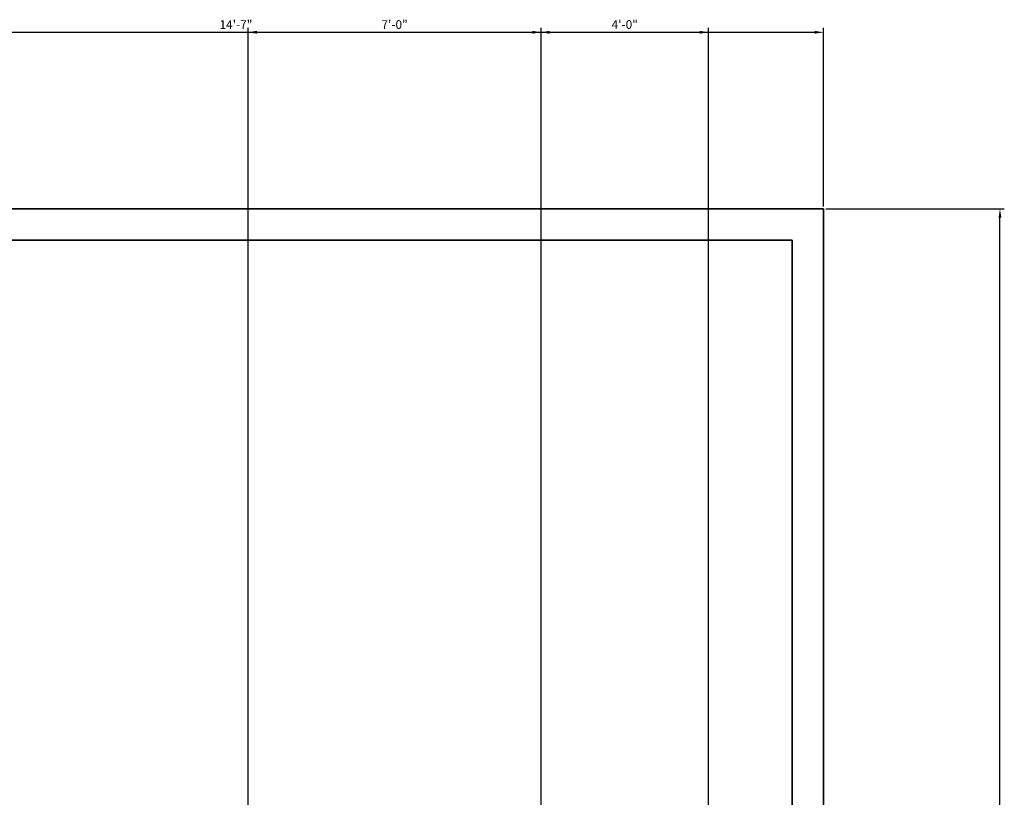
# Model space of a CAD drawing. Units: inches. Extents: x 3412 to 4225, y 13529 to 14581.
# Tile 7 of 7: x 3943 to 4225, y 14358 to 14581. Entities that reach past the tile are written whole.
import ezdxf

# ---------------------------------------------------------------- set-up
doc = ezdxf.new("R2010")
doc.units = ezdxf.units.IN
doc.layers.add('A-ANNO-DIMS', color=2, linetype='Continuous', lineweight=13)
doc.layers.add('C-SITE-WALL', color=7, linetype='Continuous', lineweight=35)
doc.styles.get("Standard").update_dxf_attribs({"font": 'arial.ttf'})
doc.dimstyles.new('ISO-25', dxfattribs={"dimtxt": 2.5, "dimasz": 2.5, "dimexe": 1.25, "dimexo": 0.625, "dimtad": 1, "dimdec": 0, "dimlunit": 3, "dimtxsty": 'Standard', "dimcen": 2.5, "dimadec": 0, "dimazin": 0, "dimtfac": 1, "dimtdec": 0, "dimtmove": 0, "dimatfit": 3, "dimfxl": 1, "dimarcsym": 0})

# ---------------------------------------------------------------- blocks, each defined once
blk = doc.blocks.new('*D56')
at = {"layer": 'A-ANNO-DIMS', "color": 0, "lineweight": -2, "transparency": 16777216}
for p, q in [((3468.36, 14527.06), (3468.36, 14578.28)), ((4173.36, 14527.06), (4173.36, 14578.28)), ((3470.86, 14577.03), (4170.86, 14577.03))]:
    blk.add_line(p, q, dxfattribs=at)
at = {"layer": 'A-ANNO-DIMS', "color": 0, "transparency": 16777216}
for points in [[(3470.86, 14577.45), (3470.86, 14576.62), (3468.36, 14577.03)], [(4170.86, 14577.45), (4170.86, 14576.62), (4173.36, 14577.03)]]:
    blk.add_solid(points, dxfattribs=at)
at = {"layer": 'Defpoints', "color": 0, "transparency": 16777216}
for p in [(4173.36, 14577.03), (3468.36, 14526.43), (4173.36, 14526.43)]:
    blk.add_point(p, dxfattribs=at)
at = {"layer": 'A-ANNO-DIMS', "color": 0, "transparency": 16777216, "insert": (3820.86, 14578.93), "char_height": 2.5, "attachment_point": 5}
blk.add_mtext('58\'-9"', dxfattribs=at)
blk = doc.blocks.new('*D57')
at = {"layer": 'A-ANNO-DIMS', "color": 0, "lineweight": -2, "transparency": 16777216}
for p, q in [((4173.98, 14526.43), (4225.21, 14526.43)), ((4223.96, 13604.93), (4223.96, 14523.93)), ((4173.98, 13602.43), (4225.21, 13602.43))]:
    blk.add_line(p, q, dxfattribs=at)
at = {"layer": 'A-ANNO-DIMS', "color": 0, "transparency": 16777216}
for points in [[(4223.54, 14523.93), (4224.37, 14523.93), (4223.96, 14526.43)], [(4223.54, 13604.93), (4224.37, 13604.93), (4223.96, 13602.43)]]:
    blk.add_solid(points, dxfattribs=at)
at = {"layer": 'Defpoints', "color": 0, "transparency": 16777216}
for p in [(4173.36, 14526.43), (4223.96, 14526.43), (4173.36, 13602.43)]:
    blk.add_point(p, dxfattribs=at)
at = {"layer": 'A-ANNO-DIMS', "color": 0, "transparency": 16777216, "insert": (4222.06, 14064.43), "char_height": 2.5, "attachment_point": 5, "rotation": 90}
blk.add_mtext('77\'-0"', dxfattribs=at)
blk = doc.blocks.new('*D72')
at = {"layer": 'A-ANNO-DIMS', "color": 0, "lineweight": -2, "transparency": 16777216}
for p, q in [((3917.36, 14353.06), (3917.36, 14578.28)), ((4092.36, 14353.06), (4092.36, 14578.28)), ((3919.86, 14577.03), (4089.86, 14577.03))]:
    blk.add_line(p, q, dxfattribs=at)
at = {"layer": 'A-ANNO-DIMS', "color": 0, "transparency": 16777216}
for points in [[(3919.86, 14577.45), (3919.86, 14576.62), (3917.36, 14577.03)], [(4089.86, 14577.45), (4089.86, 14576.62), (4092.36, 14577.03)]]:
    blk.add_solid(points, dxfattribs=at)
at = {"layer": 'Defpoints', "color": 0, "transparency": 16777216}
for p in [(4092.36, 14577.03), (3917.36, 14352.43), (4092.36, 14352.43)]:
    blk.add_point(p, dxfattribs=at)
at = {"layer": 'A-ANNO-DIMS', "color": 0, "transparency": 16777216, "insert": (4004.86, 14578.91), "char_height": 2.5, "attachment_point": 5}
blk.add_mtext('14\'-7"', dxfattribs=at)
blk = doc.blocks.new('*D83')
at = {"layer": 'A-ANNO-DIMS', "color": 0, "lineweight": -2, "transparency": 16777216}
for p, q in [((4008.36, 14044.06), (4008.36, 14578.28)), ((4092.36, 14044.06), (4092.36, 14578.28)), ((4010.86, 14577.03), (4089.86, 14577.03))]:
    blk.add_line(p, q, dxfattribs=at)
at = {"layer": 'A-ANNO-DIMS', "color": 0, "transparency": 16777216}
for points in [[(4010.86, 14577.45), (4010.86, 14576.62), (4008.36, 14577.03)], [(4089.86, 14577.45), (4089.86, 14576.62), (4092.36, 14577.03)]]:
    blk.add_solid(points, dxfattribs=at)
at = {"layer": 'Defpoints', "color": 0, "transparency": 16777216}
for p in [(4092.36, 14577.03), (4008.36, 14043.43), (4092.36, 14043.43)]:
    blk.add_point(p, dxfattribs=at)
at = {"layer": 'A-ANNO-DIMS', "color": 0, "transparency": 16777216, "insert": (4050.36, 14578.93), "char_height": 2.5, "attachment_point": 5}
blk.add_mtext('7\'-0"', dxfattribs=at)
blk = doc.blocks.new('*D84')
at = {"layer": 'A-ANNO-DIMS', "color": 0, "lineweight": -2, "transparency": 16777216}
for p, q in [((4092.36, 14044.06), (4092.36, 14578.28)), ((4140.36, 14044.06), (4140.36, 14578.28)), ((4094.86, 14577.03), (4137.86, 14577.03))]:
    blk.add_line(p, q, dxfattribs=at)
at = {"layer": 'A-ANNO-DIMS', "color": 0, "transparency": 16777216}
for points in [[(4094.86, 14577.45), (4094.86, 14576.62), (4092.36, 14577.03)], [(4137.86, 14577.45), (4137.86, 14576.62), (4140.36, 14577.03)]]:
    blk.add_solid(points, dxfattribs=at)
at = {"layer": 'Defpoints', "color": 0, "transparency": 16777216}
for p in [(4140.36, 14577.03), (4092.36, 14043.43), (4140.36, 14043.43)]:
    blk.add_point(p, dxfattribs=at)
at = {"layer": 'A-ANNO-DIMS', "color": 0, "transparency": 16777216, "insert": (4116.36, 14578.93), "char_height": 2.5, "attachment_point": 5}
blk.add_mtext('4\'-0"', dxfattribs=at)

msp = doc.modelspace()

# ---------------------------------------------------------------- linework, layer by layer
at = {"layer": 'C-SITE-WALL'}
for p, q in [((3468.36, 14526.43), (4173.36, 14526.43)), ((4173.36, 14526.43), (4173.36, 13602.43)), ((3477.36, 14517.43), (4164.36, 14517.43)), ((4164.36, 14517.43), (4164.36, 13611.43))]:
    msp.add_line(p, q, dxfattribs=at)

# ---------------------------------------------------------------- dimensions: what is measured, and where the dimension line sits
at = {"layer": 'A-ANNO-DIMS'}
for base, p1, p2, picture, middle in [((4173.36, 14577.03), (3468.36, 14526.43), (4173.36, 14526.43), '*D56', (3820.86, 14578.93)), ((4092.36, 14577.03), (3917.36, 14352.43), (4092.36, 14352.43), '*D72', (4004.86, 14578.91)), ((4092.36, 14577.03), (4008.36, 14043.43), (4092.36, 14043.43), '*D83', (4050.36, 14578.93)), ((4140.36, 14577.03), (4092.36, 14043.43), (4140.36, 14043.43), '*D84', (4116.36, 14578.93))]:
    dim = msp.add_linear_dim(base=base, p1=p1, p2=p2, dimstyle='ISO-25', override={"dimdec": 1, "dimlfac": 1, "dimrnd": 0, "dimzin": 1, "dimdsep": 46, "dimlunit": 4, "dimfrac": 2}, dxfattribs=at)
    dim.commit()
    dim.dimension.update_dxf_attribs({"geometry": picture, "text_midpoint": middle})
dim = msp.add_linear_dim(base=(4223.96, 14526.43), p1=(4173.36, 13602.43), p2=(4173.36, 14526.43), angle=90, dimstyle='ISO-25', override={"dimdec": 1, "dimlfac": 1, "dimrnd": 0, "dimzin": 1, "dimdsep": 46, "dimlunit": 4, "dimfrac": 2}, dxfattribs=at)
dim.commit()
dim.dimension.update_dxf_attribs({"geometry": '*D57', "text_midpoint": (4222.06, 14064.43)})

doc.saveas('drawing.dxf')
